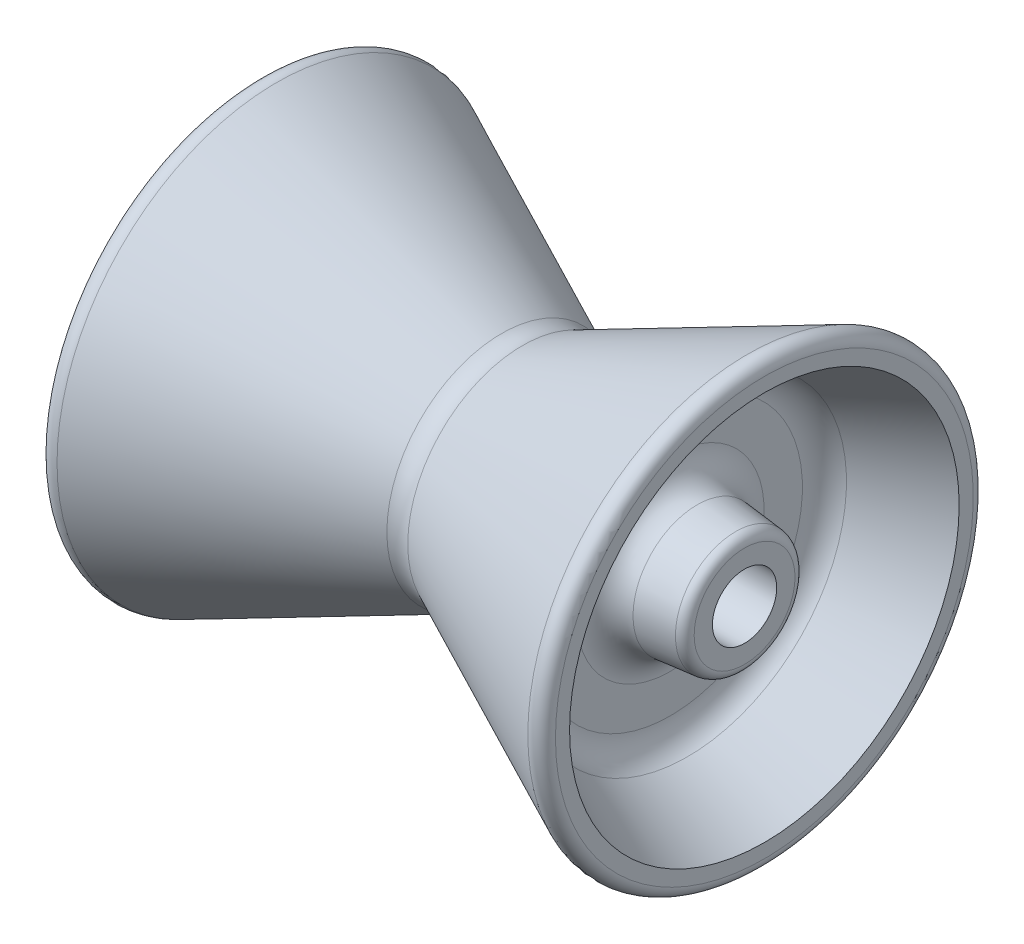
ISO-10303-21;
HEADER;
FILE_DESCRIPTION(('STEP AP214'),'2;1');
FILE_NAME('part.step','',(''),(''),'','','');
FILE_SCHEMA(('AUTOMOTIVE_DESIGN { 1 0 10303 214 1 1 1 1 }'));
ENDSEC;
DATA;
#1=APPLICATION_CONTEXT('core data for automotive mechanical design processes');
#2=APPLICATION_PROTOCOL_DEFINITION('international standard','automotive_design',2000,#1);
#3=PRODUCT_CONTEXT('',#1,'mechanical');
#4=PRODUCT('Part','Part','',(#3));
#5=PRODUCT_RELATED_PRODUCT_CATEGORY('part','',(#4));
#6=PRODUCT_DEFINITION_FORMATION('','',#4);
#7=PRODUCT_DEFINITION_CONTEXT('part definition',#1,'design');
#8=PRODUCT_DEFINITION('design','',#6,#7);
#9=PRODUCT_DEFINITION_SHAPE('','',#8);
#10=(LENGTH_UNIT() NAMED_UNIT(*) SI_UNIT(.MILLI.,.METRE.));
#11=(NAMED_UNIT(*) PLANE_ANGLE_UNIT() SI_UNIT($,.RADIAN.));
#12=(NAMED_UNIT(*) SI_UNIT($,.STERADIAN.) SOLID_ANGLE_UNIT());
#13=UNCERTAINTY_MEASURE_WITH_UNIT(LENGTH_MEASURE(1.E-05),#10,'distance_accuracy_value','');
#14=(GEOMETRIC_REPRESENTATION_CONTEXT(3) GLOBAL_UNCERTAINTY_ASSIGNED_CONTEXT((#13)) GLOBAL_UNIT_ASSIGNED_CONTEXT((#10,
#11,#12)) REPRESENTATION_CONTEXT('',''));
#15=CARTESIAN_POINT('',(0.,0.,0.));
#16=DIRECTION('',(0.,0.,1.));
#17=DIRECTION('',(1.,0.,0.));
#18=AXIS2_PLACEMENT_3D('',#15,#16,#17);
#19=CARTESIAN_POINT('',(130.,91.5196378482261,0.));
#20=DIRECTION('',(1.,0.,0.));
#21=DIRECTION('',(0.,0.,-1.));
#22=AXIS2_PLACEMENT_3D('',#19,#20,#21);
#23=PLANE('',#22);
#24=CARTESIAN_POINT('',(130.,0.,0.));
#25=DIRECTION('',(-1.,0.,0.));
#26=DIRECTION('',(0.,0.,1.));
#27=AXIS2_PLACEMENT_3D('',#24,#25,#26);
#28=CIRCLE('',#27,32.5);
#29=CARTESIAN_POINT('',(130.,0.,32.5));
#30=VERTEX_POINT('',#29);
#31=EDGE_CURVE('E10',#30,#30,#28,.T.);
#32=ORIENTED_EDGE('',*,*,#31,.F.);
#33=EDGE_LOOP('',(#32));
#34=FACE_BOUND('',#33,.T.);
#35=CARTESIAN_POINT('',(130.,0.,0.));
#36=DIRECTION('',(-1.,0.,0.));
#37=DIRECTION('',(0.,0.,1.));
#38=AXIS2_PLACEMENT_3D('',#35,#36,#37);
#39=CIRCLE('',#38,91.5196378482261);
#40=CARTESIAN_POINT('',(130.,0.,91.5196378482261));
#41=VERTEX_POINT('',#40);
#42=EDGE_CURVE('E134',#41,#41,#39,.T.);
#43=ORIENTED_EDGE('',*,*,#42,.T.);
#44=EDGE_LOOP('',(#43));
#45=FACE_BOUND('',#44,.T.);
#46=ADVANCED_FACE('F39',(#34,#45),#23,.F.);
#47=CARTESIAN_POINT('',(0.,0.,0.));
#48=DIRECTION('',(-1.,0.,0.));
#49=DIRECTION('',(0.,0.,1.));
#50=AXIS2_PLACEMENT_3D('',#47,#48,#49);
#51=CYLINDRICAL_SURFACE('',#50,32.5);
#52=CARTESIAN_POINT('',(235.,0.,0.));
#53=DIRECTION('',(-1.,0.,0.));
#54=DIRECTION('',(0.,0.,1.));
#55=AXIS2_PLACEMENT_3D('',#52,#53,#54);
#56=CIRCLE('',#55,32.5);
#57=CARTESIAN_POINT('',(235.,0.,32.5));
#58=VERTEX_POINT('',#57);
#59=EDGE_CURVE('E44',#58,#58,#56,.T.);
#60=ORIENTED_EDGE('',*,*,#59,.F.);
#61=EDGE_LOOP('',(#60));
#62=FACE_BOUND('',#61,.T.);
#63=ORIENTED_EDGE('',*,*,#31,.T.);
#64=EDGE_LOOP('',(#63));
#65=FACE_BOUND('',#64,.T.);
#66=ADVANCED_FACE('F305',(#62,#65),#51,.F.);
#67=CARTESIAN_POINT('',(235.,32.5,0.));
#68=DIRECTION('',(-1.,0.,0.));
#69=DIRECTION('',(0.,0.,1.));
#70=AXIS2_PLACEMENT_3D('',#67,#68,#69);
#71=PLANE('',#70);
#72=CARTESIAN_POINT('',(235.,0.,0.));
#73=DIRECTION('',(-1.,0.,0.));
#74=DIRECTION('',(0.,0.,1.));
#75=AXIS2_PLACEMENT_3D('',#72,#73,#74);
#76=CIRCLE('',#75,50.950124378879);
#77=CARTESIAN_POINT('',(235.,0.,50.950124378879));
#78=VERTEX_POINT('',#77);
#79=EDGE_CURVE('E47',#78,#78,#76,.T.);
#80=ORIENTED_EDGE('',*,*,#79,.F.);
#81=EDGE_LOOP('',(#80));
#82=FACE_BOUND('',#81,.T.);
#83=ORIENTED_EDGE('',*,*,#59,.T.);
#84=EDGE_LOOP('',(#83));
#85=FACE_BOUND('',#84,.T.);
#86=ADVANCED_FACE('F300',(#82,#85),#71,.F.);
#87=CARTESIAN_POINT('',(225.,0.,0.));
#88=DIRECTION('',(-1.,0.,0.));
#89=DIRECTION('',(0.,0.,1.));
#90=AXIS2_PLACEMENT_3D('',#87,#88,#89);
#91=TOROIDAL_SURFACE('',#90,50.9501243788791,10.);
#92=CARTESIAN_POINT('',(225.99503719021,0.,0.));
#93=DIRECTION('',(-1.,0.,0.));
#94=DIRECTION('',(0.,0.,1.));
#95=AXIS2_PLACEMENT_3D('',#92,#93,#94);
#96=CIRCLE('',#95,60.900496280979);
#97=CARTESIAN_POINT('',(225.99503719021,0.,60.900496280979));
#98=VERTEX_POINT('',#97);
#99=EDGE_CURVE('E52',#98,#98,#96,.T.);
#100=ORIENTED_EDGE('',*,*,#99,.F.);
#101=EDGE_LOOP('',(#100));
#102=FACE_BOUND('',#101,.T.);
#103=ORIENTED_EDGE('',*,*,#79,.T.);
#104=EDGE_LOOP('',(#103));
#105=FACE_BOUND('',#104,.T.);
#106=ADVANCED_FACE('F292',(#102,#105),#91,.T.);
#107=CARTESIAN_POINT('',(225.99503719021,0.,0.));
#108=DIRECTION('',(-1.,0.,0.));
#109=DIRECTION('',(0.,0.,1.));
#110=AXIS2_PLACEMENT_3D('',#107,#108,#109);
#111=CONICAL_SURFACE('',#110,60.900496280979,0.0996686524911619);
#112=CARTESIAN_POINT('',(187.01488842937,0.,0.));
#113=DIRECTION('',(-1.,0.,0.));
#114=DIRECTION('',(0.,0.,1.));
#115=AXIS2_PLACEMENT_3D('',#112,#113,#114);
#116=CIRCLE('',#115,64.798511157063);
#117=CARTESIAN_POINT('',(187.01488842937,0.,64.798511157063));
#118=VERTEX_POINT('',#117);
#119=EDGE_CURVE('E59',#118,#118,#116,.T.);
#120=ORIENTED_EDGE('',*,*,#119,.F.);
#121=EDGE_LOOP('',(#120));
#122=FACE_BOUND('',#121,.T.);
#123=ORIENTED_EDGE('',*,*,#99,.T.);
#124=EDGE_LOOP('',(#123));
#125=FACE_BOUND('',#124,.T.);
#126=ADVANCED_FACE('F283',(#122,#125),#111,.T.);
#127=CARTESIAN_POINT('',(190.,0.,0.));
#128=DIRECTION('',(-1.,0.,0.));
#129=DIRECTION('',(0.,0.,1.));
#130=AXIS2_PLACEMENT_3D('',#127,#128,#129);
#131=TOROIDAL_SURFACE('',#130,94.6496268633627,30.);
#132=CARTESIAN_POINT('',(160.,0.,0.));
#133=DIRECTION('',(-1.,0.,0.));
#134=DIRECTION('',(0.,0.,1.));
#135=AXIS2_PLACEMENT_3D('',#132,#133,#134);
#136=CIRCLE('',#135,94.6496268633627);
#137=CARTESIAN_POINT('',(160.,0.,94.6496268633627));
#138=VERTEX_POINT('',#137);
#139=EDGE_CURVE('E62',#138,#138,#136,.T.);
#140=ORIENTED_EDGE('',*,*,#139,.F.);
#141=EDGE_LOOP('',(#140));
#142=FACE_BOUND('',#141,.T.);
#143=ORIENTED_EDGE('',*,*,#119,.T.);
#144=EDGE_LOOP('',(#143));
#145=FACE_BOUND('',#144,.T.);
#146=ADVANCED_FACE('F276',(#142,#145),#131,.F.);
#147=CARTESIAN_POINT('',(160.,94.6496268633629,0.));
#148=DIRECTION('',(-1.,0.,0.));
#149=DIRECTION('',(0.,0.,1.));
#150=AXIS2_PLACEMENT_3D('',#147,#148,#149);
#151=PLANE('',#150);
#152=CARTESIAN_POINT('',(160.,0.,0.));
#153=DIRECTION('',(-1.,0.,0.));
#154=DIRECTION('',(0.,0.,1.));
#155=AXIS2_PLACEMENT_3D('',#152,#153,#154);
#156=CIRCLE('',#155,133.487327082176);
#157=CARTESIAN_POINT('',(160.,0.,133.487327082176));
#158=VERTEX_POINT('',#157);
#159=EDGE_CURVE('E61',#158,#158,#156,.T.);
#160=ORIENTED_EDGE('',*,*,#159,.F.);
#161=EDGE_LOOP('',(#160));
#162=FACE_BOUND('',#161,.T.);
#163=ORIENTED_EDGE('',*,*,#139,.T.);
#164=EDGE_LOOP('',(#163));
#165=FACE_BOUND('',#164,.T.);
#166=ADVANCED_FACE('F272',(#162,#165),#151,.F.);
#167=CARTESIAN_POINT('',(190.,0.,0.));
#168=DIRECTION('',(-1.,0.,0.));
#169=DIRECTION('',(0.,0.,1.));
#170=AXIS2_PLACEMENT_3D('',#167,#168,#169);
#171=TOROIDAL_SURFACE('',#170,133.487327082176,30.);
#172=CARTESIAN_POINT('',(177.321452147779,0.,0.));
#173=DIRECTION('',(-1.,0.,0.));
#174=DIRECTION('',(0.,0.,1.));
#175=AXIS2_PLACEMENT_3D('',#172,#173,#174);
#176=CIRCLE('',#175,160.676560693276);
#177=CARTESIAN_POINT('',(177.321452147779,0.,160.676560693276));
#178=VERTEX_POINT('',#177);
#179=EDGE_CURVE('E70',#178,#178,#176,.T.);
#180=ORIENTED_EDGE('',*,*,#179,.F.);
#181=EDGE_LOOP('',(#180));
#182=FACE_BOUND('',#181,.T.);
#183=ORIENTED_EDGE('',*,*,#159,.T.);
#184=EDGE_LOOP('',(#183));
#185=FACE_BOUND('',#184,.T.);
#186=ADVANCED_FACE('F270',(#182,#185),#171,.F.);
#187=CARTESIAN_POINT('',(177.321452147779,0.,0.));
#188=DIRECTION('',(1.,0.,0.));
#189=DIRECTION('',(0.,0.,-1.));
#190=AXIS2_PLACEMENT_3D('',#187,#188,#189);
#191=CONICAL_SURFACE('',#190,160.676560693276,0.436332312998581);
#192=CARTESIAN_POINT('',(255.,0.,0.));
#193=DIRECTION('',(-1.,0.,0.));
#194=DIRECTION('',(0.,0.,1.));
#195=AXIS2_PLACEMENT_3D('',#192,#193,#194);
#196=CIRCLE('',#195,196.898662431126);
#197=CARTESIAN_POINT('',(255.,0.,196.898662431126));
#198=VERTEX_POINT('',#197);
#199=EDGE_CURVE('E69',#198,#198,#196,.T.);
#200=ORIENTED_EDGE('',*,*,#199,.F.);
#201=EDGE_LOOP('',(#200));
#202=FACE_BOUND('',#201,.T.);
#203=ORIENTED_EDGE('',*,*,#179,.T.);
#204=EDGE_LOOP('',(#203));
#205=FACE_BOUND('',#204,.T.);
#206=ADVANCED_FACE('F261',(#202,#205),#191,.F.);
#207=CARTESIAN_POINT('',(255.,196.898662431126,0.));
#208=DIRECTION('',(-1.,0.,0.));
#209=DIRECTION('',(0.,0.,1.));
#210=AXIS2_PLACEMENT_3D('',#207,#208,#209);
#211=PLANE('',#210);
#212=CARTESIAN_POINT('',(255.,0.,0.));
#213=DIRECTION('',(-1.,0.,0.));
#214=DIRECTION('',(0.,0.,1.));
#215=AXIS2_PLACEMENT_3D('',#212,#213,#214);
#216=CIRCLE('',#215,211.16377307459);
#217=CARTESIAN_POINT('',(255.,0.,211.16377307459));
#218=VERTEX_POINT('',#217);
#219=EDGE_CURVE('E71',#218,#218,#216,.T.);
#220=ORIENTED_EDGE('',*,*,#219,.F.);
#221=EDGE_LOOP('',(#220));
#222=FACE_BOUND('',#221,.T.);
#223=ORIENTED_EDGE('',*,*,#199,.T.);
#224=EDGE_LOOP('',(#223));
#225=FACE_BOUND('',#224,.T.);
#226=ADVANCED_FACE('F254',(#222,#225),#211,.F.);
#227=CARTESIAN_POINT('',(243.,0.,0.));
#228=DIRECTION('',(-1.,0.,0.));
#229=DIRECTION('',(0.,0.,1.));
#230=AXIS2_PLACEMENT_3D('',#227,#228,#229);
#231=TOROIDAL_SURFACE('',#230,211.16377307459,12.);
#232=CARTESIAN_POINT('',(237.928580859112,0.,0.));
#233=DIRECTION('',(-1.,0.,0.));
#234=DIRECTION('',(0.,0.,1.));
#235=AXIS2_PLACEMENT_3D('',#232,#233,#234);
#236=CIRCLE('',#235,222.03946651903);
#237=CARTESIAN_POINT('',(237.928580859112,0.,222.03946651903));
#238=VERTEX_POINT('',#237);
#239=EDGE_CURVE('E77',#238,#238,#236,.T.);
#240=ORIENTED_EDGE('',*,*,#239,.F.);
#241=EDGE_LOOP('',(#240));
#242=FACE_BOUND('',#241,.T.);
#243=ORIENTED_EDGE('',*,*,#219,.T.);
#244=EDGE_LOOP('',(#243));
#245=FACE_BOUND('',#244,.T.);
#246=ADVANCED_FACE('F248',(#242,#245),#231,.T.);
#247=CARTESIAN_POINT('',(237.928580859112,0.,0.));
#248=DIRECTION('',(1.,0.,0.));
#249=DIRECTION('',(0.,0.,-1.));
#250=AXIS2_PLACEMENT_3D('',#247,#248,#249);
#251=CONICAL_SURFACE('',#250,222.03946651903,0.436332312998579);
#252=CARTESIAN_POINT('',(10.5654565435175,0.,0.));
#253=DIRECTION('',(-1.,0.,0.));
#254=DIRECTION('',(0.,0.,1.));
#255=AXIS2_PLACEMENT_3D('',#252,#253,#254);
#256=CIRCLE('',#255,116.018300468622);
#257=CARTESIAN_POINT('',(10.5654565435175,0.,116.018300468622));
#258=VERTEX_POINT('',#257);
#259=EDGE_CURVE('E76',#258,#258,#256,.T.);
#260=ORIENTED_EDGE('',*,*,#259,.F.);
#261=EDGE_LOOP('',(#260));
#262=FACE_BOUND('',#261,.T.);
#263=ORIENTED_EDGE('',*,*,#239,.T.);
#264=EDGE_LOOP('',(#263));
#265=FACE_BOUND('',#264,.T.);
#266=ADVANCED_FACE('F244',(#262,#265),#251,.T.);
#267=CARTESIAN_POINT('',(0.,0.,0.));
#268=DIRECTION('',(-1.,0.,0.));
#269=DIRECTION('',(0.,0.,1.));
#270=AXIS2_PLACEMENT_3D('',#267,#268,#269);
#271=TOROIDAL_SURFACE('',#270,138.675995144539,25.);
#272=CARTESIAN_POINT('',(-10.5654565435175,0.,0.));
#273=DIRECTION('',(-1.,0.,0.));
#274=DIRECTION('',(0.,0.,1.));
#275=AXIS2_PLACEMENT_3D('',#272,#273,#274);
#276=CIRCLE('',#275,116.018300468622);
#277=CARTESIAN_POINT('',(-10.5654565435175,0.,116.018300468622));
#278=VERTEX_POINT('',#277);
#279=EDGE_CURVE('E85',#278,#278,#276,.T.);
#280=ORIENTED_EDGE('',*,*,#279,.F.);
#281=EDGE_LOOP('',(#280));
#282=FACE_BOUND('',#281,.T.);
#283=ORIENTED_EDGE('',*,*,#259,.T.);
#284=EDGE_LOOP('',(#283));
#285=FACE_BOUND('',#284,.T.);
#286=ADVANCED_FACE('F240',(#282,#285),#271,.F.);
#287=CARTESIAN_POINT('',(-10.5654565435175,0.,0.));
#288=DIRECTION('',(-1.,0.,0.));
#289=DIRECTION('',(0.,0.,1.));
#290=AXIS2_PLACEMENT_3D('',#287,#288,#289);
#291=CONICAL_SURFACE('',#290,116.018300468622,0.436332312998579);
#292=CARTESIAN_POINT('',(-237.928580859111,0.,0.));
#293=DIRECTION('',(-1.,0.,0.));
#294=DIRECTION('',(0.,0.,1.));
#295=AXIS2_PLACEMENT_3D('',#292,#293,#294);
#296=CIRCLE('',#295,222.03946651903);
#297=CARTESIAN_POINT('',(-237.928580859111,0.,222.03946651903));
#298=VERTEX_POINT('',#297);
#299=EDGE_CURVE('E84',#298,#298,#296,.T.);
#300=ORIENTED_EDGE('',*,*,#299,.F.);
#301=EDGE_LOOP('',(#300));
#302=FACE_BOUND('',#301,.T.);
#303=ORIENTED_EDGE('',*,*,#279,.T.);
#304=EDGE_LOOP('',(#303));
#305=FACE_BOUND('',#304,.T.);
#306=ADVANCED_FACE('F231',(#302,#305),#291,.T.);
#307=CARTESIAN_POINT('',(-243.,0.,0.));
#308=DIRECTION('',(-1.,0.,0.));
#309=DIRECTION('',(0.,0.,1.));
#310=AXIS2_PLACEMENT_3D('',#307,#308,#309);
#311=TOROIDAL_SURFACE('',#310,211.16377307459,12.);
#312=CARTESIAN_POINT('',(-255.,0.,0.));
#313=DIRECTION('',(-1.,0.,0.));
#314=DIRECTION('',(0.,0.,1.));
#315=AXIS2_PLACEMENT_3D('',#312,#313,#314);
#316=CIRCLE('',#315,211.16377307459);
#317=CARTESIAN_POINT('',(-255.,0.,211.16377307459));
#318=VERTEX_POINT('',#317);
#319=EDGE_CURVE('E86',#318,#318,#316,.T.);
#320=ORIENTED_EDGE('',*,*,#319,.F.);
#321=EDGE_LOOP('',(#320));
#322=FACE_BOUND('',#321,.T.);
#323=ORIENTED_EDGE('',*,*,#299,.T.);
#324=EDGE_LOOP('',(#323));
#325=FACE_BOUND('',#324,.T.);
#326=ADVANCED_FACE('F223',(#322,#325),#311,.T.);
#327=CARTESIAN_POINT('',(-255.,196.898662431126,0.));
#328=DIRECTION('',(1.,0.,0.));
#329=DIRECTION('',(0.,0.,-1.));
#330=AXIS2_PLACEMENT_3D('',#327,#328,#329);
#331=PLANE('',#330);
#332=CARTESIAN_POINT('',(-255.,0.,0.));
#333=DIRECTION('',(-1.,0.,0.));
#334=DIRECTION('',(0.,0.,1.));
#335=AXIS2_PLACEMENT_3D('',#332,#333,#334);
#336=CIRCLE('',#335,196.898662431126);
#337=CARTESIAN_POINT('',(-255.,0.,196.898662431126));
#338=VERTEX_POINT('',#337);
#339=EDGE_CURVE('E93',#338,#338,#336,.T.);
#340=ORIENTED_EDGE('',*,*,#339,.F.);
#341=EDGE_LOOP('',(#340));
#342=FACE_BOUND('',#341,.T.);
#343=ORIENTED_EDGE('',*,*,#319,.T.);
#344=EDGE_LOOP('',(#343));
#345=FACE_BOUND('',#344,.T.);
#346=ADVANCED_FACE('F218',(#342,#345),#331,.F.);
#347=CARTESIAN_POINT('',(-255.,0.,0.));
#348=DIRECTION('',(-1.,0.,0.));
#349=DIRECTION('',(0.,0.,1.));
#350=AXIS2_PLACEMENT_3D('',#347,#348,#349);
#351=CONICAL_SURFACE('',#350,196.898662431126,0.436332312998581);
#352=CARTESIAN_POINT('',(-177.321452147779,0.,0.));
#353=DIRECTION('',(-1.,0.,0.));
#354=DIRECTION('',(0.,0.,1.));
#355=AXIS2_PLACEMENT_3D('',#352,#353,#354);
#356=CIRCLE('',#355,160.676560693276);
#357=CARTESIAN_POINT('',(-177.321452147779,0.,160.676560693276));
#358=VERTEX_POINT('',#357);
#359=EDGE_CURVE('E94',#358,#358,#356,.T.);
#360=ORIENTED_EDGE('',*,*,#359,.F.);
#361=EDGE_LOOP('',(#360));
#362=FACE_BOUND('',#361,.T.);
#363=ORIENTED_EDGE('',*,*,#339,.T.);
#364=EDGE_LOOP('',(#363));
#365=FACE_BOUND('',#364,.T.);
#366=ADVANCED_FACE('F213',(#362,#365),#351,.F.);
#367=CARTESIAN_POINT('',(-190.,0.,0.));
#368=DIRECTION('',(-1.,0.,0.));
#369=DIRECTION('',(0.,0.,1.));
#370=AXIS2_PLACEMENT_3D('',#367,#368,#369);
#371=TOROIDAL_SURFACE('',#370,133.487327082176,30.);
#372=CARTESIAN_POINT('',(-160.,0.,0.));
#373=DIRECTION('',(-1.,0.,0.));
#374=DIRECTION('',(0.,0.,1.));
#375=AXIS2_PLACEMENT_3D('',#372,#373,#374);
#376=CIRCLE('',#375,133.487327082176);
#377=CARTESIAN_POINT('',(-160.,0.,133.487327082176));
#378=VERTEX_POINT('',#377);
#379=EDGE_CURVE('E100',#378,#378,#376,.T.);
#380=ORIENTED_EDGE('',*,*,#379,.F.);
#381=EDGE_LOOP('',(#380));
#382=FACE_BOUND('',#381,.T.);
#383=ORIENTED_EDGE('',*,*,#359,.T.);
#384=EDGE_LOOP('',(#383));
#385=FACE_BOUND('',#384,.T.);
#386=ADVANCED_FACE('F210',(#382,#385),#371,.F.);
#387=CARTESIAN_POINT('',(-160.,94.6496268633629,0.));
#388=DIRECTION('',(1.,0.,0.));
#389=DIRECTION('',(0.,0.,-1.));
#390=AXIS2_PLACEMENT_3D('',#387,#388,#389);
#391=PLANE('',#390);
#392=CARTESIAN_POINT('',(-160.,0.,0.));
#393=DIRECTION('',(-1.,0.,0.));
#394=DIRECTION('',(0.,0.,1.));
#395=AXIS2_PLACEMENT_3D('',#392,#393,#394);
#396=CIRCLE('',#395,94.6496268633629);
#397=CARTESIAN_POINT('',(-160.,0.,94.6496268633629));
#398=VERTEX_POINT('',#397);
#399=EDGE_CURVE('E99',#398,#398,#396,.T.);
#400=ORIENTED_EDGE('',*,*,#399,.F.);
#401=EDGE_LOOP('',(#400));
#402=FACE_BOUND('',#401,.T.);
#403=ORIENTED_EDGE('',*,*,#379,.T.);
#404=EDGE_LOOP('',(#403));
#405=FACE_BOUND('',#404,.T.);
#406=ADVANCED_FACE('F203',(#402,#405),#391,.F.);
#407=CARTESIAN_POINT('',(-190.,0.,0.));
#408=DIRECTION('',(-1.,0.,0.));
#409=DIRECTION('',(0.,0.,1.));
#410=AXIS2_PLACEMENT_3D('',#407,#408,#409);
#411=TOROIDAL_SURFACE('',#410,94.6496268633627,30.);
#412=CARTESIAN_POINT('',(-187.01488842937,0.,0.));
#413=DIRECTION('',(-1.,0.,0.));
#414=DIRECTION('',(0.,0.,1.));
#415=AXIS2_PLACEMENT_3D('',#412,#413,#414);
#416=CIRCLE('',#415,64.798511157063);
#417=CARTESIAN_POINT('',(-187.01488842937,0.,64.798511157063));
#418=VERTEX_POINT('',#417);
#419=EDGE_CURVE('E103',#418,#418,#416,.T.);
#420=ORIENTED_EDGE('',*,*,#419,.F.);
#421=EDGE_LOOP('',(#420));
#422=FACE_BOUND('',#421,.T.);
#423=ORIENTED_EDGE('',*,*,#399,.T.);
#424=EDGE_LOOP('',(#423));
#425=FACE_BOUND('',#424,.T.);
#426=ADVANCED_FACE('F194',(#422,#425),#411,.F.);
#427=CARTESIAN_POINT('',(-187.01488842937,0.,0.));
#428=DIRECTION('',(1.,0.,0.));
#429=DIRECTION('',(0.,0.,-1.));
#430=AXIS2_PLACEMENT_3D('',#427,#428,#429);
#431=CONICAL_SURFACE('',#430,64.798511157063,0.0996686524911617);
#432=CARTESIAN_POINT('',(-225.99503719021,0.,0.));
#433=DIRECTION('',(-1.,0.,0.));
#434=DIRECTION('',(0.,0.,1.));
#435=AXIS2_PLACEMENT_3D('',#432,#433,#434);
#436=CIRCLE('',#435,60.900496280979);
#437=CARTESIAN_POINT('',(-225.99503719021,0.,60.900496280979));
#438=VERTEX_POINT('',#437);
#439=EDGE_CURVE('E106',#438,#438,#436,.T.);
#440=ORIENTED_EDGE('',*,*,#439,.F.);
#441=EDGE_LOOP('',(#440));
#442=FACE_BOUND('',#441,.T.);
#443=ORIENTED_EDGE('',*,*,#419,.T.);
#444=EDGE_LOOP('',(#443));
#445=FACE_BOUND('',#444,.T.);
#446=ADVANCED_FACE('F186',(#442,#445),#431,.T.);
#447=CARTESIAN_POINT('',(-225.,0.,0.));
#448=DIRECTION('',(-1.,0.,0.));
#449=DIRECTION('',(0.,0.,1.));
#450=AXIS2_PLACEMENT_3D('',#447,#448,#449);
#451=TOROIDAL_SURFACE('',#450,50.9501243788791,10.);
#452=CARTESIAN_POINT('',(-235.,0.,0.));
#453=DIRECTION('',(-1.,0.,0.));
#454=DIRECTION('',(0.,0.,1.));
#455=AXIS2_PLACEMENT_3D('',#452,#453,#454);
#456=CIRCLE('',#455,50.950124378879);
#457=CARTESIAN_POINT('',(-235.,0.,50.950124378879));
#458=VERTEX_POINT('',#457);
#459=EDGE_CURVE('E108',#458,#458,#456,.T.);
#460=ORIENTED_EDGE('',*,*,#459,.F.);
#461=EDGE_LOOP('',(#460));
#462=FACE_BOUND('',#461,.T.);
#463=ORIENTED_EDGE('',*,*,#439,.T.);
#464=EDGE_LOOP('',(#463));
#465=FACE_BOUND('',#464,.T.);
#466=ADVANCED_FACE('F181',(#462,#465),#451,.T.);
#467=CARTESIAN_POINT('',(-235.,32.5,0.));
#468=DIRECTION('',(1.,0.,0.));
#469=DIRECTION('',(0.,0.,-1.));
#470=AXIS2_PLACEMENT_3D('',#467,#468,#469);
#471=PLANE('',#470);
#472=CARTESIAN_POINT('',(-235.,0.,0.));
#473=DIRECTION('',(-1.,0.,0.));
#474=DIRECTION('',(0.,0.,1.));
#475=AXIS2_PLACEMENT_3D('',#472,#473,#474);
#476=CIRCLE('',#475,32.5);
#477=CARTESIAN_POINT('',(-235.,0.,32.5));
#478=VERTEX_POINT('',#477);
#479=EDGE_CURVE('E115',#478,#478,#476,.T.);
#480=ORIENTED_EDGE('',*,*,#479,.F.);
#481=EDGE_LOOP('',(#480));
#482=FACE_BOUND('',#481,.T.);
#483=ORIENTED_EDGE('',*,*,#459,.T.);
#484=EDGE_LOOP('',(#483));
#485=FACE_BOUND('',#484,.T.);
#486=ADVANCED_FACE('F180',(#482,#485),#471,.F.);
#487=CARTESIAN_POINT('',(0.,0.,0.));
#488=DIRECTION('',(-1.,0.,0.));
#489=DIRECTION('',(0.,0.,1.));
#490=AXIS2_PLACEMENT_3D('',#487,#488,#489);
#491=CYLINDRICAL_SURFACE('',#490,32.5);
#492=CARTESIAN_POINT('',(-130.,0.,0.));
#493=DIRECTION('',(-1.,0.,0.));
#494=DIRECTION('',(0.,0.,1.));
#495=AXIS2_PLACEMENT_3D('',#492,#493,#494);
#496=CIRCLE('',#495,32.5);
#497=CARTESIAN_POINT('',(-130.,0.,32.5));
#498=VERTEX_POINT('',#497);
#499=EDGE_CURVE('E113',#498,#498,#496,.T.);
#500=ORIENTED_EDGE('',*,*,#499,.F.);
#501=EDGE_LOOP('',(#500));
#502=FACE_BOUND('',#501,.T.);
#503=ORIENTED_EDGE('',*,*,#479,.T.);
#504=EDGE_LOOP('',(#503));
#505=FACE_BOUND('',#504,.T.);
#506=ADVANCED_FACE('F172',(#502,#505),#491,.F.);
#507=CARTESIAN_POINT('',(-130.,91.5196378482261,0.));
#508=DIRECTION('',(-1.,0.,0.));
#509=DIRECTION('',(0.,0.,1.));
#510=AXIS2_PLACEMENT_3D('',#507,#508,#509);
#511=PLANE('',#510);
#512=CARTESIAN_POINT('',(-130.,0.,0.));
#513=DIRECTION('',(-1.,0.,0.));
#514=DIRECTION('',(0.,0.,1.));
#515=AXIS2_PLACEMENT_3D('',#512,#513,#514);
#516=CIRCLE('',#515,91.5196378482261);
#517=CARTESIAN_POINT('',(-130.,0.,91.5196378482261));
#518=VERTEX_POINT('',#517);
#519=EDGE_CURVE('E119',#518,#518,#516,.T.);
#520=ORIENTED_EDGE('',*,*,#519,.F.);
#521=EDGE_LOOP('',(#520));
#522=FACE_BOUND('',#521,.T.);
#523=ORIENTED_EDGE('',*,*,#499,.T.);
#524=EDGE_LOOP('',(#523));
#525=FACE_BOUND('',#524,.T.);
#526=ADVANCED_FACE('F164',(#522,#525),#511,.F.);
#527=CARTESIAN_POINT('',(-100.,0.,0.));
#528=DIRECTION('',(-1.,0.,0.));
#529=DIRECTION('',(0.,0.,1.));
#530=AXIS2_PLACEMENT_3D('',#527,#528,#529);
#531=TOROIDAL_SURFACE('',#530,91.5196378482264,30.);
#532=CARTESIAN_POINT('',(-87.3214521477787,0.,0.));
#533=DIRECTION('',(-1.,0.,0.));
#534=DIRECTION('',(0.,0.,1.));
#535=AXIS2_PLACEMENT_3D('',#532,#533,#534);
#536=CIRCLE('',#535,118.708871459326);
#537=CARTESIAN_POINT('',(-87.3214521477787,0.,118.708871459326));
#538=VERTEX_POINT('',#537);
#539=EDGE_CURVE('E121',#538,#538,#536,.T.);
#540=ORIENTED_EDGE('',*,*,#539,.F.);
#541=EDGE_LOOP('',(#540));
#542=FACE_BOUND('',#541,.T.);
#543=ORIENTED_EDGE('',*,*,#519,.T.);
#544=EDGE_LOOP('',(#543));
#545=FACE_BOUND('',#544,.T.);
#546=ADVANCED_FACE('F157',(#542,#545),#531,.F.);
#547=CARTESIAN_POINT('',(-87.3214521477787,0.,0.));
#548=DIRECTION('',(-1.,0.,0.));
#549=DIRECTION('',(0.,0.,1.));
#550=AXIS2_PLACEMENT_3D('',#547,#548,#549);
#551=CONICAL_SURFACE('',#550,118.708871459326,0.436332312998581);
#552=CARTESIAN_POINT('',(-21.1309130870348,0.,0.));
#553=DIRECTION('',(-1.,0.,0.));
#554=DIRECTION('',(0.,0.,1.));
#555=AXIS2_PLACEMENT_3D('',#552,#553,#554);
#556=CIRCLE('',#555,87.8437161978935);
#557=CARTESIAN_POINT('',(-21.1309130870348,0.,87.8437161978935));
#558=VERTEX_POINT('',#557);
#559=EDGE_CURVE('E123',#558,#558,#556,.T.);
#560=ORIENTED_EDGE('',*,*,#559,.F.);
#561=EDGE_LOOP('',(#560));
#562=FACE_BOUND('',#561,.T.);
#563=ORIENTED_EDGE('',*,*,#539,.T.);
#564=EDGE_LOOP('',(#563));
#565=FACE_BOUND('',#564,.T.);
#566=ADVANCED_FACE('F153',(#562,#565),#551,.F.);
#567=CARTESIAN_POINT('',(0.,0.,0.));
#568=DIRECTION('',(-1.,0.,0.));
#569=DIRECTION('',(0.,0.,1.));
#570=AXIS2_PLACEMENT_3D('',#567,#568,#569);
#571=TOROIDAL_SURFACE('',#570,133.159105549726,49.9999999999998);
#572=CARTESIAN_POINT('',(21.1309130870348,0.,0.));
#573=DIRECTION('',(-1.,0.,0.));
#574=DIRECTION('',(0.,0.,1.));
#575=AXIS2_PLACEMENT_3D('',#572,#573,#574);
#576=CIRCLE('',#575,87.8437161978935);
#577=CARTESIAN_POINT('',(21.1309130870348,0.,87.8437161978935));
#578=VERTEX_POINT('',#577);
#579=EDGE_CURVE('E130',#578,#578,#576,.T.);
#580=ORIENTED_EDGE('',*,*,#579,.F.);
#581=EDGE_LOOP('',(#580));
#582=FACE_BOUND('',#581,.T.);
#583=ORIENTED_EDGE('',*,*,#559,.T.);
#584=EDGE_LOOP('',(#583));
#585=FACE_BOUND('',#584,.T.);
#586=ADVANCED_FACE('F150',(#582,#585),#571,.T.);
#587=CARTESIAN_POINT('',(21.1309130870348,0.,0.));
#588=DIRECTION('',(1.,0.,0.));
#589=DIRECTION('',(0.,0.,-1.));
#590=AXIS2_PLACEMENT_3D('',#587,#588,#589);
#591=CONICAL_SURFACE('',#590,87.8437161978935,0.436332312998581);
#592=CARTESIAN_POINT('',(87.3214521477788,0.,0.));
#593=DIRECTION('',(-1.,0.,0.));
#594=DIRECTION('',(0.,0.,1.));
#595=AXIS2_PLACEMENT_3D('',#592,#593,#594);
#596=CIRCLE('',#595,118.708871459326);
#597=CARTESIAN_POINT('',(87.3214521477788,0.,118.708871459326));
#598=VERTEX_POINT('',#597);
#599=EDGE_CURVE('E128',#598,#598,#596,.T.);
#600=ORIENTED_EDGE('',*,*,#599,.F.);
#601=EDGE_LOOP('',(#600));
#602=FACE_BOUND('',#601,.T.);
#603=ORIENTED_EDGE('',*,*,#579,.T.);
#604=EDGE_LOOP('',(#603));
#605=FACE_BOUND('',#604,.T.);
#606=ADVANCED_FACE('F143',(#602,#605),#591,.F.);
#607=CARTESIAN_POINT('',(100.,0.,0.));
#608=DIRECTION('',(-1.,0.,0.));
#609=DIRECTION('',(0.,0.,1.));
#610=AXIS2_PLACEMENT_3D('',#607,#608,#609);
#611=TOROIDAL_SURFACE('',#610,91.5196378482264,30.);
#612=ORIENTED_EDGE('',*,*,#42,.F.);
#613=EDGE_LOOP('',(#612));
#614=FACE_BOUND('',#613,.T.);
#615=ORIENTED_EDGE('',*,*,#599,.T.);
#616=EDGE_LOOP('',(#615));
#617=FACE_BOUND('',#616,.T.);
#618=ADVANCED_FACE('F137',(#614,#617),#611,.F.);
#619=CLOSED_SHELL('',(#46,#66,#86,#106,#126,#146,#166,#186,#206,#226,#246,#266,#286,#306,#326,
#346,#366,#386,#406,#426,#446,#466,#486,#506,#526,#546,#566,#586,#606,#618));
#620=MANIFOLD_SOLID_BREP('B2',#619);
#621=ADVANCED_BREP_SHAPE_REPRESENTATION('',(#18,#620),#14);
#622=SHAPE_DEFINITION_REPRESENTATION(#9,#621);
ENDSEC;
END-ISO-10303-21;
